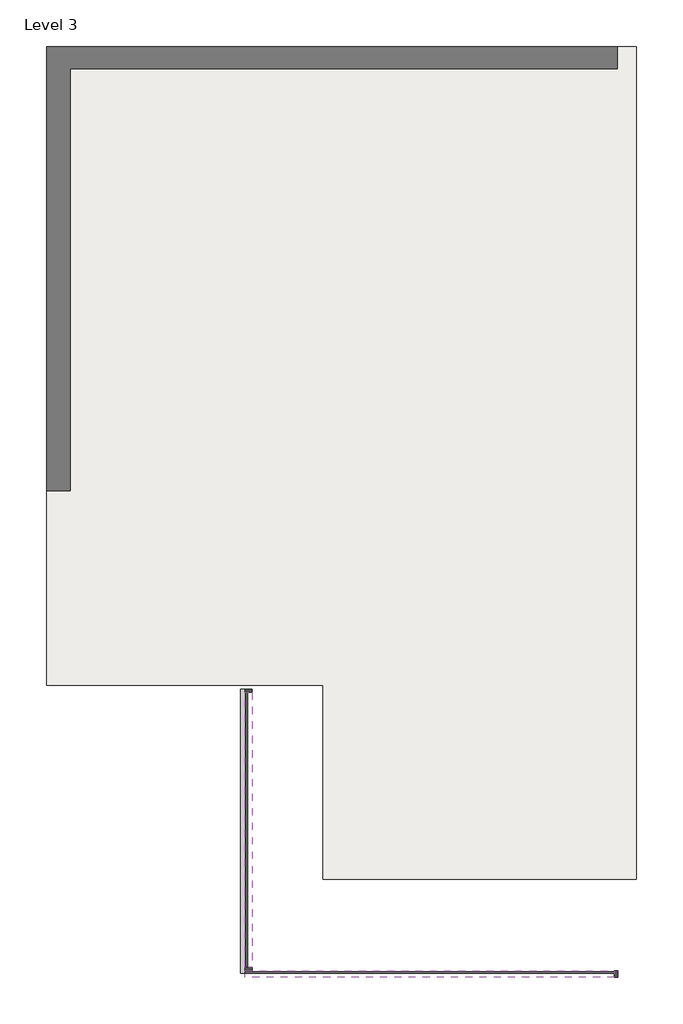
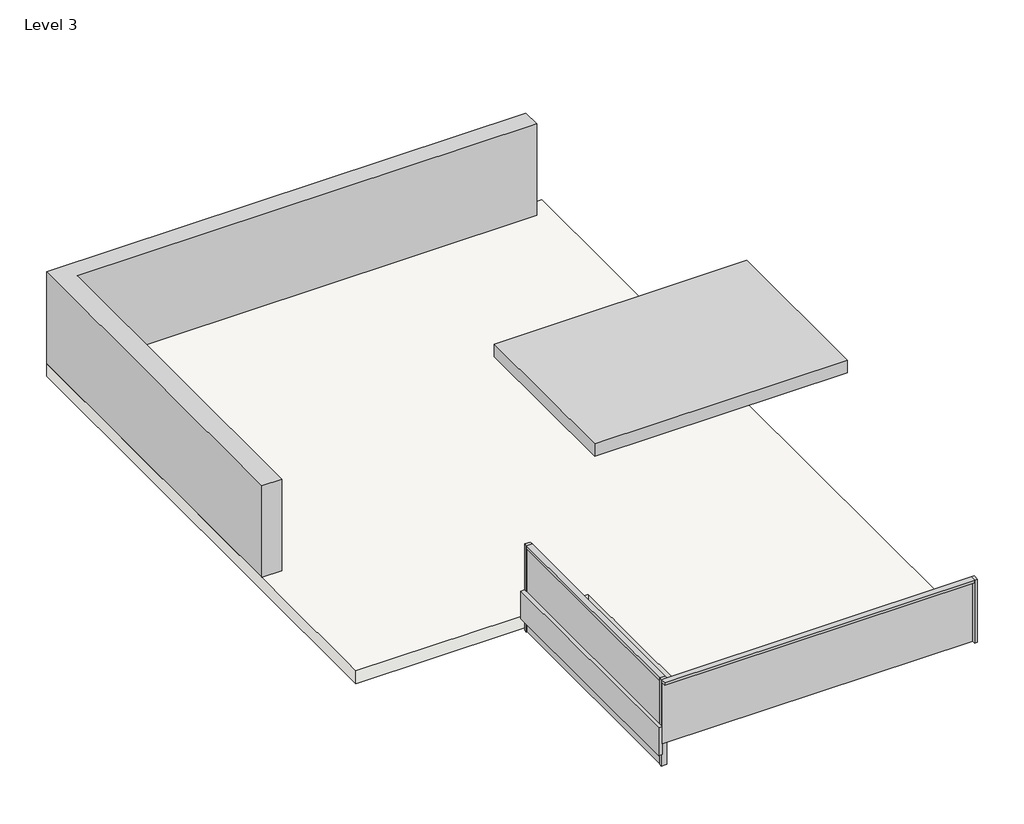
# One storey: 5 members, 2 plates, 2 proxies, 1 roof.
"""IFC4 building model written with IfcOpenShell, lengths in millimetres."""

from ifc_helpers import new_model, si_unit, frame, origin, place, context, project, spatial, polyline, outline, extrude, transform, mapped, element, save
from components import generic_models_8_generic_models_8_3e5e579e, generic_models_9_generic_models_9_df2407d9, member_2b438bbf, member_0c2b78d7, member_9c0893e9, member_b399a46d, system_panel_glazed_5985f842, system_panel_glazed_95ff72d9

model = new_model("IFC4")

# Units and contexts
model_context = context("Model", 3, world=origin())
ifc_project = project(units=[si_unit("LENGTHUNIT", "METRE", prefix="MILLI")], contexts=[model_context])

# Site, building, storey
site = spatial("IfcSite", under=ifc_project)
building = spatial("IfcBuilding", under=site)
storey = spatial("IfcBuildingStorey", under=building, Name="Level 3", Elevation=6096.0)

# Proxies
placement = place(None, origin())
generic_models_8_generic_models_8_shape = generic_models_8_generic_models_8_3e5e579e(model_context)
element("IfcBuildingElementProxy", 1, Name="Generic Models 8 : Generic Models 8", ObjectType="Generic Models 8 : Generic Models 8", at=placement, inside=storey, context=model_context, shape_type="MappedRepresentation", body=[
    mapped(generic_models_8_generic_models_8_shape, transform((0.0, 0.0, 0.0), x_axis=(1.0, 0.0, 0.0), y_axis=(0.0, 1.0, 0.0), z_axis=(0.0, 0.0, 1.0))),
])
generic_models_9_generic_models_9_shape = generic_models_9_generic_models_9_df2407d9(model_context)
element("IfcBuildingElementProxy", 2, Name="Generic Models 9 : Generic Models 9", ObjectType="Generic Models 9 : Generic Models 9", at=placement, inside=storey, context=model_context, shape_type="MappedRepresentation", body=[
    mapped(generic_models_9_generic_models_9_shape, transform((0.0, 0.0, 0.0), x_axis=(1.0, 0.0, 0.0), y_axis=(0.0, 1.0, 0.0), z_axis=(0.0, 0.0, 1.0))),
])

# Members
member_shape = member_2b438bbf(model_context)
element("IfcMember", 3, ObjectType="Rectangular Mullion : 2.5\" x 5\" rectangular", at=placement, inside=storey, context=model_context, shape_type="MappedRepresentation", body=[
    mapped(member_shape, transform((-5162.1527592, -14850.2902495, 8150.3954044), x_axis=(0.0, 0.0, 1.0), y_axis=(0.0, -1.0, 0.0), z_axis=(1.0, 0.0, 0.0))),
])
member_2_shape = member_0c2b78d7(model_context)
element("IfcMember", 4, ObjectType="Rectangular Mullion : 2.5\" x 5\" rectangular", at=placement, inside=storey, context=model_context, shape_type="MappedRepresentation", body=[
    mapped(member_2_shape, transform((-5098.6527592, -14850.2902495, 6651.0332234), x_axis=(1.0, 0.0, 0.0), y_axis=(0.0, -1.0, 0.0), z_axis=(0.0, 0.0, -1.0))),
])
member_3_shape = member_9c0893e9(model_context)
element("IfcMember", 5, ObjectType="Rectangular Mullion : 2.5\" x 5\" rectangular", at=placement, inside=storey, context=model_context, shape_type="MappedRepresentation", body=[
    mapped(member_3_shape, transform((-12065.4471301, -9540.1468404, 8150.3954044), x_axis=(0.0, 0.0, 1.0), y_axis=(1.0, 0.0, 0.0), z_axis=(0.0, 1.0, 0.0))),
])
member_4_shape = member_b399a46d(model_context)
element("IfcMember", 6, ObjectType="Rectangular Mullion : 2.5\" x 5\" rectangular", at=placement, inside=storey, context=model_context, shape_type="MappedRepresentation", body=[
    mapped(member_4_shape, transform((-12065.4471301, -14786.7902495, 8150.3954044), x_axis=(0.0, -1.0, 0.0), y_axis=(1.0, 0.0, 0.0), z_axis=(0.0, 0.0, 1.0))),
])
element("IfcMember", 7, ObjectType="Rectangular Mullion : 2.5\" x 5\" rectangular", at=placement, inside=storey, context=model_context, shape_type="MappedRepresentation", body=[
    mapped(member_4_shape, transform((-12065.4471301, -9476.6468404, 6096.0), x_axis=(0.0, 1.0, 0.0), y_axis=(1.0, 0.0, 0.0), z_axis=(0.0, 0.0, -1.0))),
])

# Plates
system_panel_glazed_shape = system_panel_glazed_5985f842(model_context)
element("IfcPlate", 8, ObjectType="System Panel : Glazed", at=placement, inside=storey, context=model_context, shape_type="MappedRepresentation", body=[
    mapped(system_panel_glazed_shape, transform((-8645.5499447, -14850.2902495, 6651.0332234), x_axis=(1.0, 0.0, 0.0), y_axis=(0.0, 1.0, 0.0), z_axis=(0.0, 0.0, 1.0))),
])
system_panel_glazed_2_shape = system_panel_glazed_95ff72d9(model_context)
element("IfcPlate", 9, ObjectType="System Panel : Glazed", at=placement, inside=storey, context=model_context, shape_type="MappedRepresentation", body=[
    mapped(system_panel_glazed_2_shape, transform((-12065.4471301, -12131.7185449, 6096.0), x_axis=(0.0, 1.0, 0.0), y_axis=(-1.0, 0.0, 0.0), z_axis=(0.0, 0.0, 1.0))),
])

# Roof
element("IfcRoof", 10, ObjectType="Generic - 12\"", at=placement, inside=storey, context=model_context, shape_type="SweptSolid", body=[
    extrude(outline(polyline([(-15877.1321088, 2639.1531596), (-4751.9321088, 2639.1531596), (-4751.9321088, -13058.0468404), (-10657.4321088, -13058.0468404), (-10657.4321088, -9400.4468404), (-15877.1321088, -9400.4468404), (-15877.1321088, 2639.1531596)])), frame((0.0, 0.0, 6096.0), z_axis=(0.0, 0.0, 1.0), x_axis=(1.0, 0.0, 0.0)), (0.0, 0.0, 1.0), 304.8),
])

save(model, "model.ifc")

# Revit data of these elements
# Type "Rectangular Mullion : 2.5\" x 5\" rectangular"
#   built-in parameter 1007304 = 0.416667 (stored number, unit not read)
#   built-in parameter 1007301 = 0.104167 (stored number, unit not read)
#   built-in parameter 1007300 = 0.104167 (stored number, unit not read)
# Type "System Panel : Glazed"
#   Construction Type Id = "GSP4R"
#   Analytic Construction = "1/8 in Pilkington single glazing"
#   Visual Light Transmittance = 0.9
#   Solar Heat Gain Coefficient = 0.86
#   Heat Transfer Coefficient (U) = 1.18115 BTU/(h·ft²·°F)
#   Define Thermal Properties by = 1
# Type "Generic - 12\""
#   Assembly Code = "B1020"
#   Layers, outside or top first: 1' - 0" no material (function 1)
# Element 1 (IfcBuildingElementProxy, "Generic Models 8 : Generic Models 8")
#   Phase Created = New Construction
# Element 2 (IfcBuildingElementProxy, "Generic Models 9 : Generic Models 9")
#   Phase Created = New Construction
# Elements 3, 4, 5, 6, 7 (IfcMember, "Rectangular Mullion : 2.5\" x 5\" rectangular")
#   Phase Created = New Construction
#   Materials on its faces: "Aluminum"
# Elements 8, 9 (IfcPlate, "System Panel : Glazed")
#   Phase Created = New Construction
#   Materials on its faces: "Glass"
# Element 10 (IfcRoof, "Generic - 12\"")
#   built-in parameter 1001705 = 21 (stored number, unit not read)
#   built-in parameter 1001710 = 33615
#   Phase Created = New Construction
#   Materials on its faces: "Default Roof"
# Materials
#   "Aluminum": class "Metal", colour RGB 247 247 247, transparency 0, Description = "Aluminum 6061", Cost = 0
#   "Glass": class "Glass", colour RGB 0 128 192, transparency 0.75, Description = "Soda Lime Glass", Cost = 0
#   "Default Roof": colour RGB 88 101 114, transparency 0, Cost = 0
